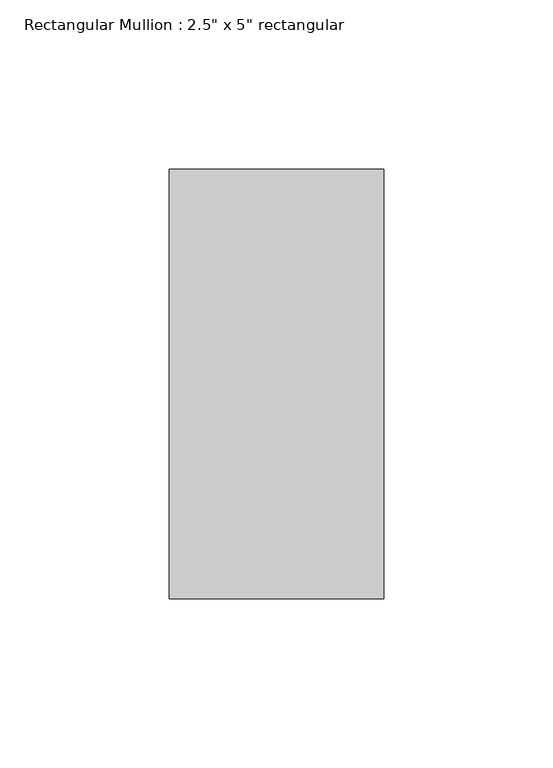
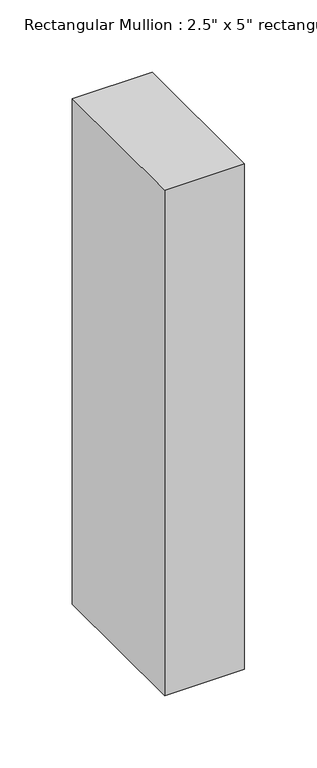
"""IFC4 building model written with IfcOpenShell, lengths in millimetres: member geometry."""

from ifc_helpers import new_model, si_unit, frame, origin, place, context, project, spatial, polyline, outline, extrude, source, transform, mapped, element, save


def member_70b87a21(model_context):
    return source(origin(), model_context, "Body", "SweptSolid", [
        extrude(outline(polyline([(31.75, 63.5), (31.75, -63.5), (-31.75, -63.5), (-31.75, 63.5), (31.75, 63.5)])), frame((0.0, 0.0, -425.45), z_axis=(0.0, 0.0, 1.0), x_axis=(1.0, 0.0, 0.0)), (0.0, 0.0, 1.0), 425.45),
    ])


if __name__ == "__main__":
    model = new_model("IFC4")
    model_context = context("Model", 3, world=origin())
    ifc_project = project(units=[si_unit("LENGTHUNIT", "METRE", prefix="MILLI")], contexts=[model_context])
    site = spatial("IfcSite", under=ifc_project)
    building = spatial("IfcBuilding", under=site)
    placement = place(None, origin())
    member_shape = member_70b87a21(model_context)
    element("IfcMember", 1, ObjectType="Rectangular Mullion : 2.5\" x 5\" rectangular", at=placement, inside=building, context=model_context, shape_type="MappedRepresentation", body=[
        mapped(member_shape, transform((0.0, 0.0, 0.0), x_axis=(1.0, 0.0, 0.0), y_axis=(0.0, 1.0, 0.0), z_axis=(0.0, 0.0, 1.0))),
    ])
    save(model, "model.ifc")

# Revit data of these elements
# Type "Rectangular Mullion : 2.5\" x 5\" rectangular"
#   built-in parameter 1007304 = 0.416667 (stored number, unit not read)
#   built-in parameter 1007301 = 0.104167 (stored number, unit not read)
#   built-in parameter 1007300 = 0.104167 (stored number, unit not read)
# Element 1 (IfcMember, "Rectangular Mullion : 2.5\" x 5\" rectangular")
#   Materials on its faces: "Aluminum"
# Materials
#   "Aluminum": class "Metal", colour RGB 247 247 247, transparency 0, Description = "Aluminum 6061", Cost = 0
